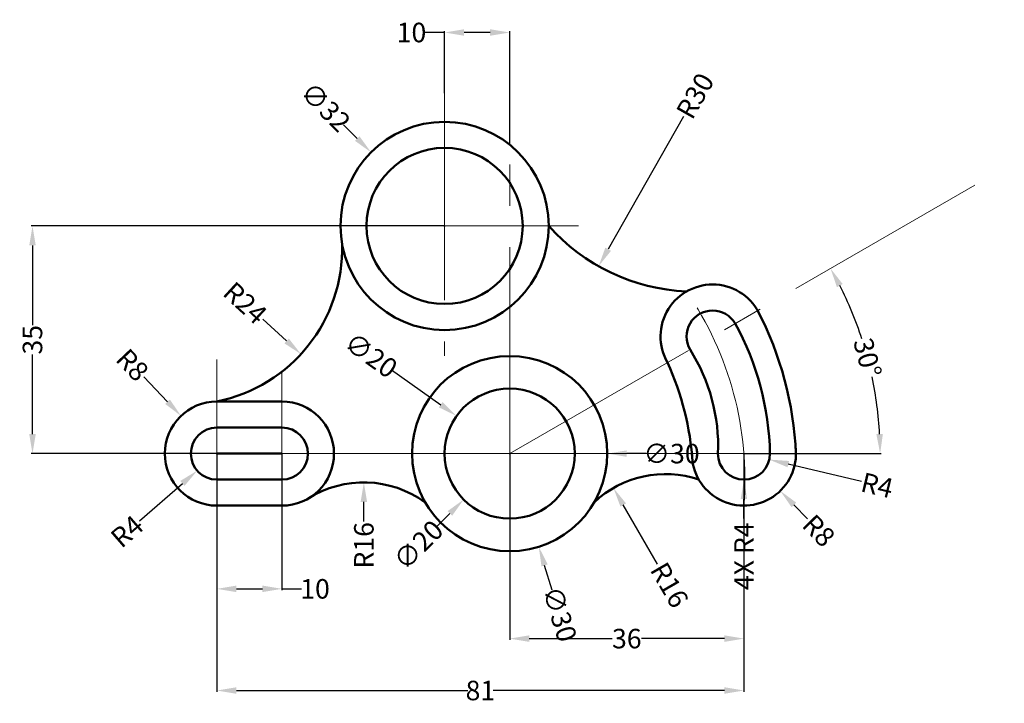
# Model space of a CAD drawing. Units: millimetres. Extents: x 224 to 375, y 68 to 173.
import ezdxf

# ---------------------------------------------------------------- set-up
doc = ezdxf.new("R2010")
doc.units = ezdxf.units.MM
doc.header["$MEASUREMENT"] = 0
doc.linetypes.add('CENTER', pattern=[50.8, 31.75, -6.35, 6.35, -6.35])
for name, color, linetype, lineweight in [('M-CNTR', 1, 'CENTER', 18), ('M-CONS', 8, 'Continuous', 13), ('M-DIMS', 2, 'Continuous', 25), ('M-OUTL', 7, 'Continuous', 50)]:
    doc.layers.add(name, color=color, linetype=linetype, lineweight=lineweight)
doc.styles.get("Standard").update_dxf_attribs({"font": 'arial.ttf'})
doc.dimstyles.get("Standard").update_dxf_attribs({"dimtxt": 3, "dimasz": 3, "dimexe": 0.18, "dimexo": 0.0625, "dimgap": 0.09, "dimtad": 0, "dimdec": 0, "dimzin": 0, "dimdsep": 46, "dimtxsty": 'Standard', "dimcen": 0.09, "dimadec": 0, "dimazin": 0, "dimtfac": 1, "dimtdec": 0, "dimtofl": 0, "dimtmove": 0, "dimatfit": 3, "dimfxl": 1, "dimtolj": 1, "dimtzin": 0, "dimarcsym": 0})

# ---------------------------------------------------------------- blocks, each defined once
blk = doc.blocks.new('*D1')
at = {"layer": 'Defpoints', "color": 0, "transparency": 16777216}
for p in [(253.84, 106.65), (334.84, 106.65), (334.84, 70.23)]:
    blk.add_point(p, dxfattribs=at)
at = {"layer": 'M-DIMS', "color": 0, "lineweight": -2, "transparency": 16777216}
for p, q in [((253.84, 106.59), (253.84, 70.05)), ((334.84, 106.59), (334.84, 70.05)), ((256.84, 70.23), (292.39, 70.23)), ((331.84, 70.23), (296.29, 70.23))]:
    blk.add_line(p, q, dxfattribs=at)
at = {"layer": 'M-DIMS', "color": 0, "transparency": 16777216}
for points in [[(256.84, 70.73), (256.84, 69.73), (253.84, 70.23)], [(331.84, 70.73), (331.84, 69.73), (334.84, 70.23)]]:
    blk.add_solid(points, dxfattribs=at)
at = {"layer": 'M-DIMS', "color": 0, "transparency": 16777216, "insert": (294.34, 70.23), "char_height": 3, "attachment_point": 5}
blk.add_mtext('\\A1;81', dxfattribs=at)
blk = doc.blocks.new('*D2')
at = {"layer": 'Defpoints', "color": 0, "transparency": 16777216}
for p in [(288.84, 141.65), (225.51, 106.65), (253.84, 106.65)]:
    blk.add_point(p, dxfattribs=at)
at = {"layer": 'M-DIMS', "color": 0, "lineweight": -2, "transparency": 16777216}
for p, q in [((288.78, 141.65), (225.33, 141.65)), ((225.51, 138.65), (225.51, 126.4)), ((225.51, 109.65), (225.51, 121.9)), ((253.78, 106.65), (225.33, 106.65))]:
    blk.add_line(p, q, dxfattribs=at)
at = {"layer": 'M-DIMS', "color": 0, "transparency": 16777216}
for points in [[(225.01, 138.65), (226.01, 138.65), (225.51, 141.65)], [(225.01, 109.65), (226.01, 109.65), (225.51, 106.65)]]:
    blk.add_solid(points, dxfattribs=at)
at = {"layer": 'M-DIMS', "color": 0, "transparency": 16777216, "insert": (225.51, 124.15), "char_height": 3, "attachment_point": 5, "rotation": 90}
blk.add_mtext('\\A1;35', dxfattribs=at)
blk = doc.blocks.new('*D3')
at = {"layer": 'Defpoints', "color": 0, "transparency": 16777216}
for p in [(298.84, 106.65), (334.84, 106.65), (334.84, 78.21)]:
    blk.add_point(p, dxfattribs=at)
at = {"layer": 'M-DIMS', "color": 0, "lineweight": -2, "transparency": 16777216}
for p, q in [((298.84, 106.59), (298.84, 78.03)), ((334.84, 106.59), (334.84, 78.03)), ((301.84, 78.21), (314.61, 78.21)), ((331.84, 78.21), (319.08, 78.21))]:
    blk.add_line(p, q, dxfattribs=at)
at = {"layer": 'M-DIMS', "color": 0, "transparency": 16777216}
for points in [[(301.84, 78.71), (301.84, 77.71), (298.84, 78.21)], [(331.84, 78.71), (331.84, 77.71), (334.84, 78.21)]]:
    blk.add_solid(points, dxfattribs=at)
at = {"layer": 'M-DIMS', "color": 0, "transparency": 16777216, "insert": (316.84, 78.21), "char_height": 3, "attachment_point": 5}
blk.add_mtext('\\A1;36', dxfattribs=at)
blk = doc.blocks.new('*D4')
at = {"layer": 'Defpoints', "color": 0, "transparency": 16777216}
for p in [(253.84, 106.65), (263.84, 106.65), (263.84, 85.86)]:
    blk.add_point(p, dxfattribs=at)
at = {"layer": 'M-DIMS', "color": 0, "lineweight": -2, "transparency": 16777216}
for p, q in [((253.84, 106.59), (253.84, 85.68)), ((263.84, 106.59), (263.84, 85.68)), ((256.84, 85.86), (260.84, 85.86)), ((263.84, 85.86), (266.84, 85.86))]:
    blk.add_line(p, q, dxfattribs=at)
at = {"layer": 'M-DIMS', "color": 0, "transparency": 16777216}
for points in [[(256.84, 86.36), (256.84, 85.36), (253.84, 85.86)], [(260.84, 86.36), (260.84, 85.36), (263.84, 85.86)]]:
    blk.add_solid(points, dxfattribs=at)
at = {"layer": 'M-DIMS', "color": 0, "transparency": 16777216, "insert": (268.93, 85.86), "char_height": 3, "attachment_point": 5}
blk.add_mtext('\\A1;10', dxfattribs=at)
blk = doc.blocks.new('*D5')
at = {"layer": 'Defpoints', "color": 0, "transparency": 16777216}
for p in [(288.84, 171.39), (288.84, 162), (298.84, 154.14)]:
    blk.add_point(p, dxfattribs=at)
at = {"layer": 'M-DIMS', "color": 0, "lineweight": -2, "transparency": 16777216}
for p, q in [((288.84, 171.39), (285.84, 171.39)), ((288.84, 162.06), (288.84, 171.57)), ((295.84, 171.39), (291.84, 171.39)), ((298.84, 154.21), (298.84, 171.57))]:
    blk.add_line(p, q, dxfattribs=at)
at = {"layer": 'M-DIMS', "color": 0, "transparency": 16777216}
for points in [[(291.84, 171.89), (291.84, 170.89), (288.84, 171.39)], [(295.84, 171.89), (295.84, 170.89), (298.84, 171.39)]]:
    blk.add_solid(points, dxfattribs=at)
at = {"layer": 'M-DIMS', "color": 0, "transparency": 16777216, "insert": (283.75, 171.39), "char_height": 3, "attachment_point": 5}
blk.add_mtext('\\A1;10', dxfattribs=at)
blk = doc.blocks.new('*D6')
at = {"layer": 'Defpoints', "color": 0, "transparency": 16777216}
for p in [(374.85, 150.54), (354.91, 116.54), (253.84, 106.65), (298.84, 106.65), (334.84, 106.65)]:
    blk.add_point(p, dxfattribs=at)
at = {"layer": 'M-DIMS', "color": 0, "lineweight": -2, "transparency": 16777216}
blk.add_line((334.9, 106.65), (355.95, 106.65), dxfattribs=at)
for start, end in [(18.0527, 26.9803), (3.0197, 11.9473)]:
    blk.add_arc((298.84, 106.65), 56.93, start, end, dxfattribs=at)
at = {"layer": 'M-DIMS', "color": 0, "transparency": 16777216}
for points in [[(349.13, 132.24), (350.01, 132.72), (348.14, 135.12)], [(356.19, 109.67), (355.19, 109.64), (355.77, 106.65)]]:
    blk.add_solid(points, dxfattribs=at)
at = {"layer": 'M-DIMS', "color": 0, "transparency": 16777216, "insert": (353.83, 121.39), "char_height": 3, "attachment_point": 5, "rotation": 285}
blk.add_mtext('\\A1;30°', dxfattribs=at)
blk = doc.blocks.new('*D7')
at = {"layer": 'Defpoints', "color": 0, "transparency": 16777216}
for p in [(327.29, 161.56), (312.5, 135.46)]:
    blk.add_point(p, dxfattribs=at)
at = {"layer": 'M-DIMS', "color": 0, "lineweight": -2, "transparency": 16777216}
blk.add_line((325.53, 158.46), (313.98, 138.07), dxfattribs=at)
at = {"layer": 'M-DIMS', "color": 0, "transparency": 16777216}
blk.add_solid([(313.54, 138.31), (314.41, 137.82), (312.5, 135.46)], dxfattribs=at)
at = {"layer": 'M-DIMS', "color": 0, "transparency": 16777216, "insert": (327.34, 161.65), "char_height": 3, "attachment_point": 5, "rotation": 60.4558}
blk.add_mtext('\\A1;R30', dxfattribs=at)
blk = doc.blocks.new('*D8')
at = {"layer": 'Defpoints', "color": 0, "transparency": 16777216}
for p in [(276.43, 102.22), (276.43, 86.22)]:
    blk.add_point(p, dxfattribs=at)
at = {"layer": 'M-DIMS', "color": 0, "lineweight": -2, "transparency": 16777216}
blk.add_line((276.43, 96.22), (276.43, 99.22), dxfattribs=at)
at = {"layer": 'M-DIMS', "color": 0, "transparency": 16777216}
blk.add_solid([(275.93, 99.22), (276.93, 99.22), (276.43, 102.22)], dxfattribs=at)
at = {"layer": 'M-DIMS', "color": 0, "transparency": 16777216, "insert": (276.43, 92.55), "char_height": 3, "attachment_point": 5, "rotation": 90}
blk.add_mtext('\\A1;R16', dxfattribs=at)
blk = doc.blocks.new('*D9')
at = {"layer": 'Defpoints', "color": 0, "transparency": 16777216}
for p in [(314.79, 101.35), (322.79, 87.5)]:
    blk.add_point(p, dxfattribs=at)
at = {"layer": 'M-DIMS', "color": 0, "lineweight": -2, "transparency": 16777216}
blk.add_line((321.56, 89.63), (316.29, 98.75), dxfattribs=at)
at = {"layer": 'M-DIMS', "color": 0, "transparency": 16777216}
blk.add_solid([(316.72, 99), (315.86, 98.5), (314.79, 101.35)], dxfattribs=at)
at = {"layer": 'M-DIMS', "color": 0, "transparency": 16777216, "insert": (323.4, 86.45), "char_height": 3, "attachment_point": 5, "rotation": 300}
blk.add_mtext('\\A1;R16', dxfattribs=at)
blk = doc.blocks.new('*D10')
at = {"layer": 'Defpoints', "color": 0, "transparency": 16777216}
for p in [(334.84, 106.65), (338.73, 105.73)]:
    blk.add_point(p, dxfattribs=at)
at = {"layer": 'M-DIMS', "color": 0, "lineweight": -2, "transparency": 16777216}
for p, q in [((334.75, 106.65), (334.93, 106.65)), ((334.84, 106.56), (334.84, 106.74)), ((352.88, 102.36), (341.65, 105.03))]:
    blk.add_line(p, q, dxfattribs=at)
at = {"layer": 'M-DIMS', "color": 0, "transparency": 16777216}
blk.add_solid([(341.77, 105.52), (341.54, 104.55), (338.73, 105.73)], dxfattribs=at)
at = {"layer": 'M-DIMS', "color": 0, "transparency": 16777216, "insert": (355.31, 101.78), "char_height": 3, "attachment_point": 5, "rotation": 346.5994}
blk.add_mtext('\\A1;R4', dxfattribs=at)
blk = doc.blocks.new('*D11')
at = {"layer": 'Defpoints', "color": 0, "transparency": 16777216}
for p in [(290.68, 112.44), (307, 100.87)]:
    blk.add_point(p, dxfattribs=at)
at = {"layer": 'M-DIMS', "color": 0, "lineweight": -2, "transparency": 16777216}
for p, q in [((280.68, 119.53), (288.24, 114.17)), ((298.75, 106.65), (298.93, 106.65)), ((298.84, 106.56), (298.84, 106.74))]:
    blk.add_line(p, q, dxfattribs=at)
at = {"layer": 'M-DIMS', "color": 0, "transparency": 16777216}
blk.add_solid([(288.53, 114.58), (287.95, 113.76), (290.68, 112.44)], dxfattribs=at)
at = {"layer": 'M-DIMS', "color": 0, "transparency": 16777216, "insert": (277.53, 121.77), "char_height": 3, "attachment_point": 5, "rotation": 324.6635}
blk.add_mtext('\\A1;∅20', dxfattribs=at)
blk = doc.blocks.new('*D12')
at = {"layer": 'Defpoints', "color": 0, "transparency": 16777216}
for p in [(294.37, 120.97), (303.31, 92.33)]:
    blk.add_point(p, dxfattribs=at)
at = {"layer": 'M-DIMS', "color": 0, "lineweight": -2, "transparency": 16777216}
for p, q in [((298.75, 106.65), (298.93, 106.65)), ((298.84, 106.56), (298.84, 106.74)), ((305.39, 85.67), (304.2, 89.47))]:
    blk.add_line(p, q, dxfattribs=at)
at = {"layer": 'M-DIMS', "color": 0, "transparency": 16777216}
blk.add_solid([(304.68, 89.62), (303.73, 89.32), (303.31, 92.33)], dxfattribs=at)
at = {"layer": 'M-DIMS', "color": 0, "transparency": 16777216, "insert": (306.54, 81.98), "char_height": 3, "attachment_point": 5, "rotation": 287.3279}
blk.add_mtext('\\A1;∅30', dxfattribs=at)
blk = doc.blocks.new('*D13')
at = {"layer": 'Defpoints', "color": 0, "transparency": 16777216}
for p in [(249.09, 138.18), (266.77, 121.94)]:
    blk.add_point(p, dxfattribs=at)
at = {"layer": 'M-DIMS', "color": 0, "lineweight": -2, "transparency": 16777216}
blk.add_line((260.9, 127.33), (264.56, 123.97), dxfattribs=at)
at = {"layer": 'M-DIMS', "color": 0, "transparency": 16777216}
blk.add_solid([(264.9, 124.34), (264.22, 123.6), (266.77, 121.94)], dxfattribs=at)
at = {"layer": 'M-DIMS', "color": 0, "transparency": 16777216, "insert": (258.2, 129.81), "char_height": 3, "attachment_point": 5, "rotation": 317.4252}
blk.add_mtext('\\A1;R24', dxfattribs=at)
blk = doc.blocks.new('*D14')
at = {"layer": 'Defpoints', "color": 0, "transparency": 16777216}
for p in [(248.33, 112.45), (253.84, 106.65)]:
    blk.add_point(p, dxfattribs=at)
at = {"layer": 'M-DIMS', "color": 0, "lineweight": -2, "transparency": 16777216}
for p, q in [((242.6, 118.46), (246.26, 114.62)), ((253.75, 106.65), (253.93, 106.65)), ((253.84, 106.56), (253.84, 106.74))]:
    blk.add_line(p, q, dxfattribs=at)
at = {"layer": 'M-DIMS', "color": 0, "transparency": 16777216}
blk.add_solid([(246.62, 114.97), (245.9, 114.28), (248.33, 112.45)], dxfattribs=at)
at = {"layer": 'M-DIMS', "color": 0, "transparency": 16777216, "insert": (240.87, 120.28), "char_height": 3, "attachment_point": 5, "rotation": 313.5914}
blk.add_mtext('\\A1;R8', dxfattribs=at)
blk = doc.blocks.new('*D15')
at = {"layer": 'Defpoints', "color": 0, "transparency": 16777216}
for p in [(253.84, 106.65), (250.82, 104.03)]:
    blk.add_point(p, dxfattribs=at)
at = {"layer": 'M-DIMS', "color": 0, "lineweight": -2, "transparency": 16777216}
for p, q in [((253.75, 106.65), (253.93, 106.65)), ((253.84, 106.56), (253.84, 106.74)), ((241.93, 96.33), (248.55, 102.07))]:
    blk.add_line(p, q, dxfattribs=at)
at = {"layer": 'M-DIMS', "color": 0, "transparency": 16777216}
blk.add_solid([(248.23, 102.45), (248.88, 101.69), (250.82, 104.03)], dxfattribs=at)
at = {"layer": 'M-DIMS', "color": 0, "transparency": 16777216, "insert": (240.04, 94.69), "char_height": 3, "attachment_point": 5, "rotation": 40.9314}
blk.add_mtext('\\A1;R4', dxfattribs=at)
blk = doc.blocks.new('*D16')
at = {"layer": 'Defpoints', "color": 0, "transparency": 16777216}
for p in [(334.84, 106.65), (340.42, 100.92)]:
    blk.add_point(p, dxfattribs=at)
at = {"layer": 'M-DIMS', "color": 0, "lineweight": -2, "transparency": 16777216}
for p, q in [((334.75, 106.65), (334.93, 106.65)), ((334.84, 106.56), (334.84, 106.74)), ((344.6, 96.62), (342.51, 98.77))]:
    blk.add_line(p, q, dxfattribs=at)
at = {"layer": 'M-DIMS', "color": 0, "transparency": 16777216}
blk.add_solid([(342.87, 99.12), (342.15, 98.42), (340.42, 100.92)], dxfattribs=at)
at = {"layer": 'M-DIMS', "color": 0, "transparency": 16777216, "insert": (346.35, 94.81), "char_height": 3, "attachment_point": 5, "rotation": 314.1919}
blk.add_mtext('\\A1;R8', dxfattribs=at)
blk = doc.blocks.new('*D17')
at = {"layer": 'Defpoints', "color": 0, "transparency": 16777216}
for p in [(277.53, 152.97), (300.15, 130.34)]:
    blk.add_point(p, dxfattribs=at)
at = {"layer": 'M-DIMS', "color": 0, "lineweight": -2, "transparency": 16777216}
for p, q in [((273.29, 157.21), (275.41, 155.09)), ((288.75, 141.65), (288.93, 141.65)), ((288.84, 141.56), (288.84, 141.74))]:
    blk.add_line(p, q, dxfattribs=at)
at = {"layer": 'M-DIMS', "color": 0, "transparency": 16777216}
blk.add_solid([(275.76, 155.44), (275.06, 154.74), (277.53, 152.97)], dxfattribs=at)
at = {"layer": 'M-DIMS', "color": 0, "transparency": 16777216, "insert": (270.56, 159.94), "char_height": 3, "attachment_point": 5, "rotation": 314.9894}
blk.add_mtext('\\A1;∅32', dxfattribs=at)
blk = doc.blocks.new('*D18')
at = {"layer": 'Defpoints', "color": 0, "transparency": 16777216}
for p in [(305.91, 113.73), (291.77, 99.58)]:
    blk.add_point(p, dxfattribs=at)
at = {"layer": 'M-DIMS', "color": 0, "lineweight": -2, "transparency": 16777216}
for p, q in [((298.75, 106.65), (298.93, 106.65)), ((298.84, 106.56), (298.84, 106.74)), ((287.53, 95.34), (289.65, 97.46))]:
    blk.add_line(p, q, dxfattribs=at)
at = {"layer": 'M-DIMS', "color": 0, "transparency": 16777216}
blk.add_solid([(289.3, 97.81), (290, 97.11), (291.77, 99.58)], dxfattribs=at)
at = {"layer": 'M-DIMS', "color": 0, "transparency": 16777216, "insert": (284.8, 92.6), "char_height": 3, "attachment_point": 5, "rotation": 45.0073}
blk.add_mtext('\\A1;∅20', dxfattribs=at)
blk = doc.blocks.new('*D19')
at = {"layer": 'Defpoints', "color": 0, "transparency": 16777216}
for p in [(334.84, 106.65), (334.84, 102.65)]:
    blk.add_point(p, dxfattribs=at)
at = {"layer": 'M-DIMS', "color": 0, "lineweight": -2, "transparency": 16777216}
for p, q in [((334.75, 106.65), (334.93, 106.65)), ((334.84, 106.56), (334.84, 106.74)), ((334.84, 96.65), (334.84, 99.65))]:
    blk.add_line(p, q, dxfattribs=at)
at = {"layer": 'M-DIMS', "color": 0, "transparency": 16777216}
blk.add_solid([(334.34, 99.65), (335.34, 99.65), (334.84, 102.65)], dxfattribs=at)
at = {"layer": 'M-DIMS', "color": 0, "transparency": 16777216, "insert": (334.84, 90.87), "char_height": 3, "attachment_point": 5, "rotation": 90}
blk.add_mtext('\\A1;4X R4', dxfattribs=at)
blk = doc.blocks.new('*D20')
at = {"layer": 'Defpoints', "color": 0, "transparency": 16777216}
for p in [(283.84, 106.65), (313.84, 106.65)]:
    blk.add_point(p, dxfattribs=at)
at = {"layer": 'M-DIMS', "color": 0, "lineweight": -2, "transparency": 16777216}
for p, q in [((298.75, 106.65), (298.93, 106.65)), ((298.84, 106.56), (298.84, 106.74)), ((319.84, 106.65), (316.84, 106.65))]:
    blk.add_line(p, q, dxfattribs=at)
at = {"layer": 'M-DIMS', "color": 0, "transparency": 16777216}
blk.add_solid([(316.84, 107.15), (316.84, 106.15), (313.84, 106.65)], dxfattribs=at)
at = {"layer": 'M-DIMS', "color": 0, "transparency": 16777216, "insert": (323.71, 106.65), "char_height": 3, "attachment_point": 5, "rotation": 0.0007}
blk.add_mtext('\\A1;∅30', dxfattribs=at)

msp = doc.modelspace()

# ---------------------------------------------------------------- linework, layer by layer
at = {"layer": 'M-CNTR'}
for p, q in [((288.84, 162), (288.84, 121.69)), ((298.84, 106.65), (298.84, 154.14)), ((298.84, 106.65), (374.85, 150.54)), ((309.44, 141.65), (270.8, 141.65)), ((298.84, 124), (298.84, 85.02)), ((253.84, 121.14), (253.84, 83.65)), ((263.84, 119.25), (263.84, 84.41)), ((245.84, 106.65), (342.84, 106.65))]:
    msp.add_line(p, q, dxfattribs=at)
msp.add_arc((283.91, 102.65), 51.09, 355.5091, 34.4909, dxfattribs=at)
at = {"layer": 'M-CONS'}
msp.add_line((253.84, 106.65), (334.84, 106.65), dxfattribs=at)
at = {"layer": 'M-OUTL'}
for p, q in [((253.84, 114.65), (263.84, 114.65)), ((253.84, 110.65), (263.84, 110.65)), ((253.84, 106.65), (263.84, 106.65)), ((253.84, 102.65), (263.84, 102.65)), ((253.84, 98.65), (263.84, 98.65))]:
    msp.add_line(p, q, dxfattribs=at)
for centre, radius in [((288.84, 141.65), 16), ((288.84, 141.65), 12), ((298.84, 106.65), 15), ((298.84, 106.65), 10)]:
    msp.add_circle(centre, radius, dxfattribs=at)
for centre, radius, start, end in [((327.29, 161.56), 30, 221.5577, 267.5705), ((249.09, 138.18), 24, 281.4084, 1.6675), ((330.02, 124.65), 8, 23.9844, 210), ((330.02, 124.65), 4, 30, 210), ((290.06, 104.3), 52.83, 2.5525, 27.4475), ((295.52, 105.77), 43.33, 1.1755, 28.8245), ((303.15, 107.81), 27.72, 357.614, 32.386), ((282.48, 102.27), 44.58, 3.929, 24.355), ((253.84, 106.65), 8, 90, 270), ((263.84, 106.65), 8, 270, 90), ((253.84, 106.65), 4, 90, 270), ((263.84, 106.65), 4, 270, 90), ((334.84, 106.65), 8, 180, 6.0156), ((334.84, 106.65), 4, 180, 0), ((322.79, 87.5), 16, 71.3272, 133.2298), ((276.43, 86.22), 16, 53.9121, 122.4509), ((322.9, 72.87), 28.43, 65.0627, 65.1603)]:
    msp.add_arc(centre, radius, start, end, dxfattribs=at)

# ---------------------------------------------------------------- dimensions: what is measured, and where the dimension line sits
at = {"layer": 'M-DIMS'}
for base, p1, p2, picture, middle in [((288.84, 171.39), (298.84, 154.14), (288.84, 162), '*D5', (283.75, 171.39)), ((334.84, 70.23), (253.84, 106.65), (334.84, 106.65), '*D1', (294.34, 70.23)), ((263.84, 85.86), (253.84, 106.65), (263.84, 106.65), '*D4', (268.93, 85.86)), ((334.84, 78.21), (298.84, 106.65), (334.84, 106.65), '*D3', (316.84, 78.21))]:
    dim = msp.add_linear_dim(base=base, p1=p1, p2=p2, dimstyle='Standard', override={"dimclrd": 0, "dimclre": 0, "dimclrt": 0}, dxfattribs=at)
    dim.commit()
    dim.dimension.update_dxf_attribs({"geometry": picture, "text_midpoint": middle})
for center, mpoint, picture, middle in [((327.29, 161.56), (312.5, 135.46), '*D7', (327.34, 161.65)), ((249.09, 138.18), (266.77, 121.94), '*D13', (258.2, 129.81)), ((253.84, 106.65), (248.33, 112.45), '*D14', (240.87, 120.28)), ((253.84, 106.65), (250.82, 104.03), '*D15', (240.04, 94.69)), ((334.84, 106.65), (338.73, 105.73), '*D10', (355.31, 101.78)), ((276.43, 86.22), (276.43, 102.22), '*D8', (276.43, 92.55)), ((322.79, 87.5), (314.79, 101.35), '*D9', (323.4, 86.45))]:
    dim = msp.add_radius_dim(center=center, mpoint=mpoint, dimstyle='Standard', override={"dimclrd": 0, "dimclre": 0, "dimclrt": 0}, dxfattribs=at)
    dim.commit()
    dim.dimension.update_dxf_attribs({"geometry": picture, "text_midpoint": middle, "dimtype": 164})
for p1, p2, override, picture, middle in [((300.15, 130.34), (277.53, 152.97), {"dimdec": 0, "dimlfac": 1, "dimrnd": 0, "dimzin": 0, "dimdsep": 46, "dimlunit": 2}, '*D17', (270.56, 159.94)), ((307, 100.87), (290.68, 112.44), {"dimclrd": 0, "dimclre": 0, "dimclrt": 0}, '*D11', (277.53, 121.77)), ((294.37, 120.97), (303.31, 92.33), {"dimclrd": 0, "dimclre": 0, "dimclrt": 0}, '*D12', (306.54, 81.98))]:
    dim = msp.add_diameter_dim_2p(p1=p1, p2=p2, dimstyle='Standard', override=override, dxfattribs=at)
    dim.commit()
    dim.dimension.update_dxf_attribs({"geometry": picture, "text_midpoint": middle, "dimtype": 163})
dim = msp.add_angular_dim_2l(base=(354.91, 116.54), line1=((253.84, 106.65), (334.84, 106.65)), line2=((298.84, 106.65), (374.85, 150.54)), dimstyle='Standard', override={"dimclrd": 0, "dimclre": 0, "dimclrt": 0}, dxfattribs=at)
dim.commit()
dim.dimension.update_dxf_attribs({"geometry": '*D6', "text_midpoint": (353.83, 121.39)})
dim = msp.add_linear_dim(base=(225.51, 106.65), p1=(288.84, 141.65), p2=(253.84, 106.65), angle=90, dimstyle='Standard', override={"dimclrd": 0, "dimclre": 0, "dimclrt": 0}, dxfattribs=at)
dim.commit()
dim.dimension.update_dxf_attribs({"geometry": '*D2', "text_midpoint": (225.51, 124.15)})
for p1, p2, picture, middle in [((305.91, 113.73), (291.77, 99.58), '*D18', (284.8, 92.6)), ((283.84, 106.65), (313.84, 106.65), '*D20', (323.71, 106.65))]:
    dim = msp.add_diameter_dim_2p(p1=p1, p2=p2, dimstyle='Standard', override={"dimdec": 0, "dimlfac": 1, "dimrnd": 0, "dimzin": 0, "dimdsep": 46, "dimlunit": 2}, dxfattribs=at)
    dim.commit()
    dim.dimension.update_dxf_attribs({"geometry": picture, "text_midpoint": middle})
dim = msp.add_radius_dim(center=(334.84, 106.65), mpoint=(334.84, 102.65), text='4X <>', dimstyle='Standard', override={"dimdec": 0, "dimlfac": 1, "dimrnd": 0, "dimzin": 0, "dimdsep": 46, "dimlunit": 2}, dxfattribs=at)
dim.commit()
dim.dimension.update_dxf_attribs({"geometry": '*D19', "text_midpoint": (334.84, 90.87)})
dim = msp.add_radius_dim(center=(334.84, 106.65), mpoint=(340.42, 100.92), dimstyle='Standard', override={"dimclrd": 0, "dimclre": 0, "dimclrt": 0}, dxfattribs=at)
dim.commit()
dim.dimension.update_dxf_attribs({"geometry": '*D16', "text_midpoint": (346.35, 94.81)})

doc.saveas('drawing.dxf')
